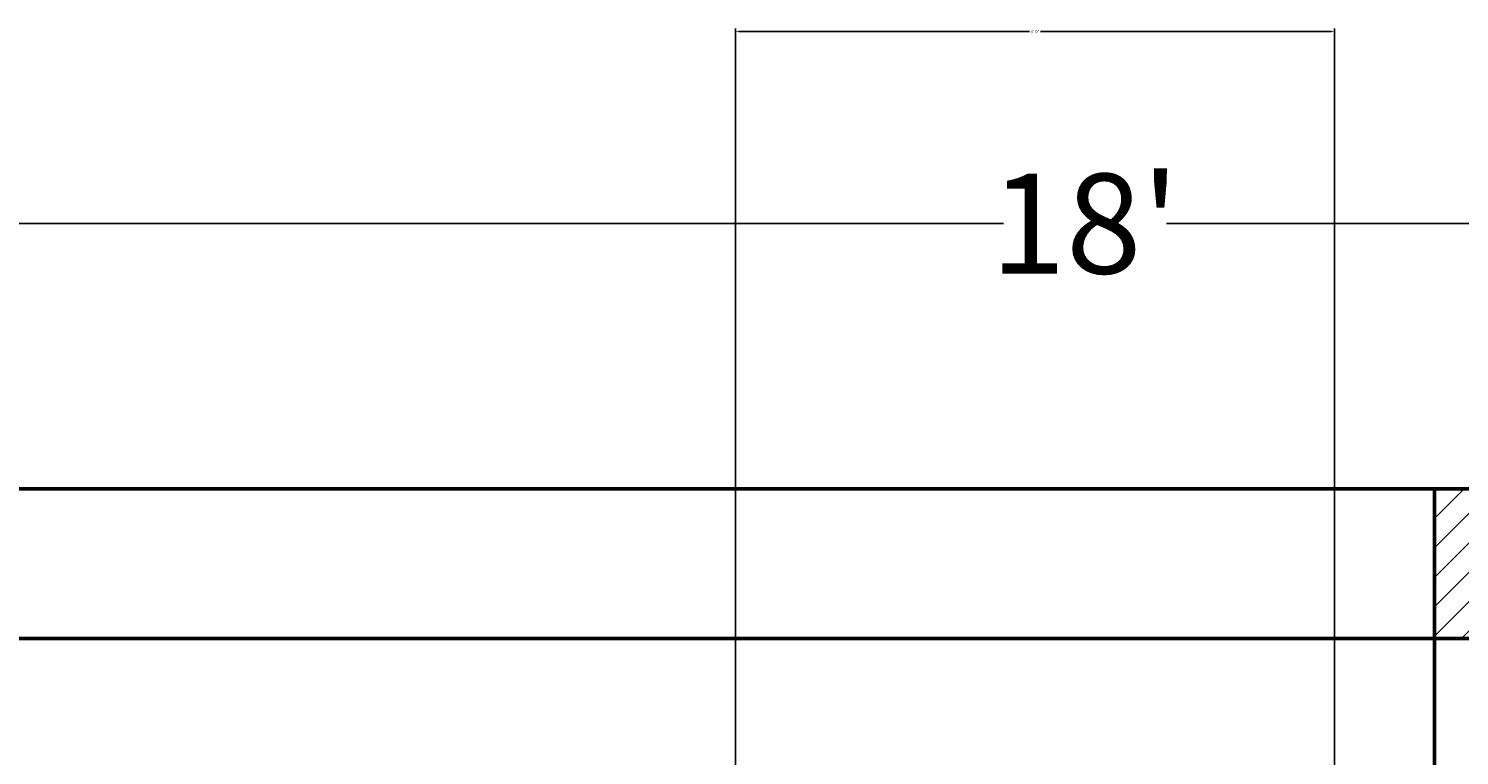
# Model space of a CAD drawing. Units: inches. Extents: x 0 to 281, y -535 to 46.
# Tile 21 of 22: x 72 to 158, y 3 to 46. Entities that reach past the tile are written whole.
import ezdxf

# ---------------------------------------------------------------- set-up
doc = ezdxf.new("R2010")
doc.units = ezdxf.units.IN
doc.header["$MEASUREMENT"] = 0
for name, color, linetype, lineweight in [('A-ANNO-DIMS', 2, 'Continuous', 18), ('A-COLS-PATT', 152, 'Continuous', 13), ('A-WALL', 7, 'Continuous', 50)]:
    doc.layers.add(name, color=color, linetype=linetype, lineweight=lineweight)
doc.styles.get("Standard").update_dxf_attribs({"font": 'arial.ttf'})
doc.dimstyles.get("Standard").update_dxf_attribs({"dimtxt": 0.18, "dimasz": 0.18, "dimexe": 0.18, "dimexo": 0.0625, "dimgap": 0.09, "dimtad": 0, "dimtih": 1, "dimtoh": 1, "dimdec": 0, "dimzin": 0, "dimdsep": 46, "dimlunit": 3, "dimtxsty": 'Standard', "dimcen": 0.09, "dimadec": 0, "dimazin": 0, "dimtfac": 1, "dimtdec": 0, "dimtofl": 0, "dimtmove": 0, "dimatfit": 3, "dimfxl": 1, "dimtolj": 1, "dimtzin": 0, "dimarcsym": 0})

# ---------------------------------------------------------------- blocks, each defined once
blk = doc.blocks.new('*D17')
at = {"layer": 'A-ANNO-DIMS', "color": 0, "lineweight": -2, "transparency": 16777216}
for p, q in [((27.459, 18.652), (27.459, 34.691)), ((27.639, 34.511), (130.56, 34.511)), ((243.279, 34.511), (140.358, 34.511)), ((243.459, 18.652), (243.459, 34.691))]:
    blk.add_line(p, q, dxfattribs=at)
at = {"layer": 'A-ANNO-DIMS', "color": 0, "transparency": 16777216}
for points in [[(27.639, 34.541), (27.639, 34.481), (27.459, 34.511)], [(243.279, 34.541), (243.279, 34.481), (243.459, 34.511)]]:
    blk.add_solid(points, dxfattribs=at)
at = {"layer": 'Defpoints', "color": 0, "transparency": 16777216}
for p in [(243.459, 34.511), (27.459, 18.589), (243.459, 18.589)]:
    blk.add_point(p, dxfattribs=at)
at = {"layer": 'A-ANNO-DIMS', "color": 0, "transparency": 16777216, "insert": (135.459, 34.511), "char_height": 6, "attachment_point": 5}
blk.add_mtext("\\A1;18'", dxfattribs=at)
blk = doc.blocks.new('*D45')
at = {"layer": 'A-ANNO-DIMS', "color": 0, "lineweight": -2, "transparency": 16777216}
for p, q in [((114.459, -263.348), (114.459, 46.219)), ((114.639, 46.039), (132.13, 46.039)), ((150.279, 46.039), (132.788, 46.039)), ((150.459, -263.348), (150.459, 46.219))]:
    blk.add_line(p, q, dxfattribs=at)
at = {"layer": 'A-ANNO-DIMS', "color": 0, "transparency": 16777216}
for points in [[(114.639, 46.069), (114.639, 46.009), (114.459, 46.039)], [(150.279, 46.069), (150.279, 46.009), (150.459, 46.039)]]:
    blk.add_solid(points, dxfattribs=at)
at = {"layer": 'Defpoints', "color": 0, "transparency": 16777216}
for p in [(150.459, 46.039), (114.459, -263.411), (150.459, -263.411)]:
    blk.add_point(p, dxfattribs=at)
at = {"layer": 'A-ANNO-DIMS', "color": 0, "transparency": 16777216, "insert": (132.459, 46.039), "char_height": 0.18, "attachment_point": 5}
blk.add_mtext('\\A1;3\'-0"', dxfattribs=at)
blk = doc.blocks.new('*D47')
at = {"layer": 'A-ANNO-DIMS', "color": 0, "lineweight": -2, "transparency": 16777216}
for p, q in [((114.459, -392.348), (114.459, 46.219)), ((114.639, 46.039), (132.13, 46.039)), ((150.279, 46.039), (132.788, 46.039)), ((150.459, -392.348), (150.459, 46.219))]:
    blk.add_line(p, q, dxfattribs=at)
at = {"layer": 'A-ANNO-DIMS', "color": 0, "transparency": 16777216}
for points in [[(114.639, 46.069), (114.639, 46.009), (114.459, 46.039)], [(150.279, 46.069), (150.279, 46.009), (150.459, 46.039)]]:
    blk.add_solid(points, dxfattribs=at)
at = {"layer": 'Defpoints', "color": 0, "transparency": 16777216}
for p in [(150.459, 46.039), (114.459, -392.411), (150.459, -392.411)]:
    blk.add_point(p, dxfattribs=at)
at = {"layer": 'A-ANNO-DIMS', "color": 0, "transparency": 16777216, "insert": (132.459, 46.039), "char_height": 0.18, "attachment_point": 5}
blk.add_mtext('\\A1;3\'-0"', dxfattribs=at)

msp = doc.modelspace()

# ---------------------------------------------------------------- hatches: boundary and pattern name
at = {"layer": 'A-COLS-PATT'}
h = msp.add_hatch(dxfattribs=at)
h.set_pattern_fill('ANSI31', color=256, scale=10)
h.paths.add_polyline_path([(36.459, 18.589), (27.459, 18.589), (27.459, 9.589), (36.459, 9.589)])
h.paths.add_polyline_path([(165.459, 18.589), (156.459, 18.589), (156.459, 9.589), (165.459, 9.589)])
h.paths.add_polyline_path([(243.459, 18.589), (234.459, 18.589), (234.459, 9.589), (243.459, 9.589)])
h.paths.add_polyline_path([(243.459, -122.411), (234.459, -122.411), (234.459, -131.411), (243.459, -131.411)])
h.paths.add_polyline_path([(36.459, -122.411), (27.459, -122.411), (27.459, -131.411), (36.459, -131.411)])
h.paths.add_polyline_path([(36.459, -498.411), (27.459, -498.411), (27.459, -507.411), (36.459, -507.411)])
h.paths.add_polyline_path([(243.459, -498.411), (234.459, -498.411), (234.459, -507.411), (243.459, -507.411)])
h.paths.add_polyline_path([(159.459, -498.411), (150.459, -498.411), (150.459, -507.411), (159.459, -507.411)])
h.paths.add_polyline_path([(36.459, -392.411), (27.459, -392.411), (27.459, -401.411), (36.459, -401.411)])
h.paths.add_polyline_path([(159.459, -392.411), (150.459, -392.411), (150.459, -401.411), (159.459, -401.411)])
h.paths.add_polyline_path([(243.459, -392.411), (234.459, -392.411), (234.459, -401.411), (243.459, -401.411)])
h.paths.add_polyline_path([(36.459, -263.411), (27.459, -263.411), (27.459, -272.411), (36.459, -272.411)])
h.paths.add_polyline_path([(243.459, -263.411), (234.459, -263.411), (234.459, -272.411), (243.459, -272.411)])

# ---------------------------------------------------------------- linework, layer by layer
at = {"layer": 'A-WALL'}
for p, q in [((27.459, 18.589), (243.459, 18.589)), ((156.459, 18.589), (156.459, -131.411)), ((27.459, 9.589), (243.459, 9.589))]:
    msp.add_line(p, q, dxfattribs=at)

# ---------------------------------------------------------------- dimensions: what is measured, and where the dimension line sits
at = {"layer": 'A-ANNO-DIMS'}
for base, p1, p2, override, picture, middle in [((150.459, 46.039), (114.459, -263.411), (150.459, -263.411), {"dimdec": 1, "dimlfac": 1, "dimrnd": 0, "dimzin": 1, "dimdsep": 46, "dimlunit": 4, "dimfrac": 2}, '*D45', (132.459, 46.039)), ((150.459, 46.039), (114.459, -392.411), (150.459, -392.411), {"dimdec": 1, "dimlfac": 1, "dimrnd": 0, "dimzin": 1, "dimdsep": 46, "dimlunit": 4, "dimfrac": 2}, '*D47', (132.459, 46.039)), ((243.459, 34.511), (27.459, 18.589), (243.459, 18.589), {"dimtxt": 6, "dimclrd": 0, "dimclre": 0, "dimclrt": 0}, '*D17', (135.459, 34.511))]:
    dim = msp.add_linear_dim(base=base, p1=p1, p2=p2, dimstyle='Standard', override=override, dxfattribs=at)
    dim.commit()
    dim.dimension.update_dxf_attribs({"geometry": picture, "text_midpoint": middle})

doc.saveas('drawing.dxf')
